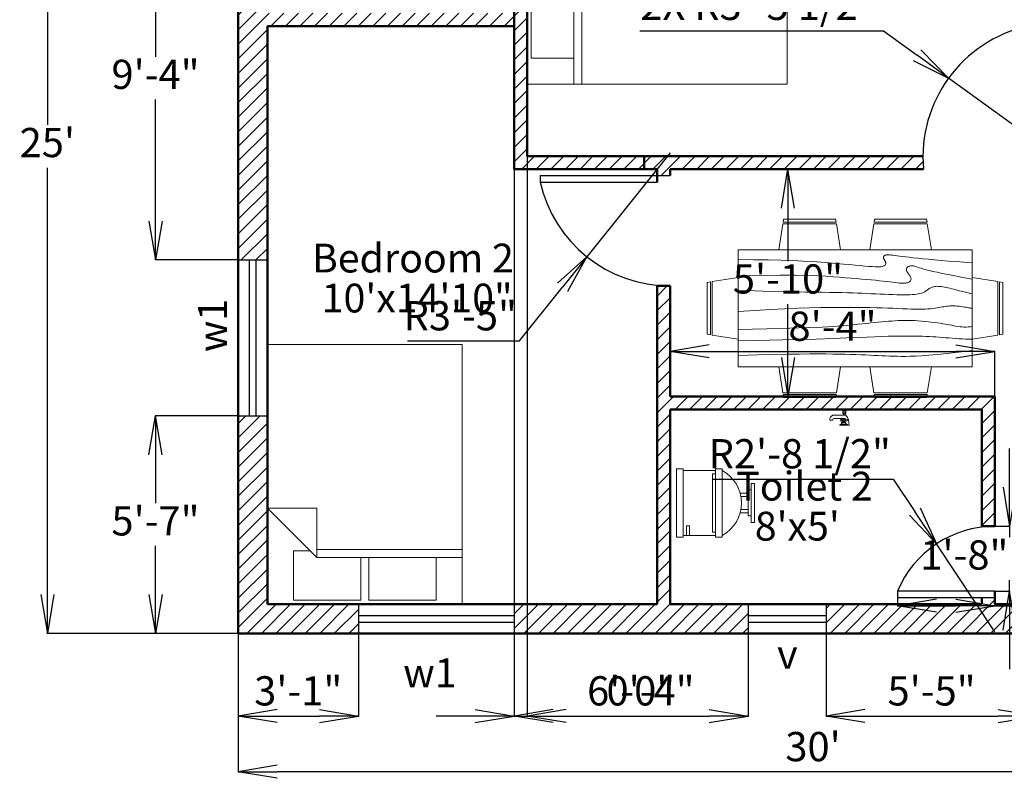
# Model space of a CAD drawing. Units: inches. Extents: x 1856 to 3350, y 1624 to 2224.
# Tile 1 of 7: x 1856 to 2159, y 1782 to 2016. Entities that reach past the tile are written whole.
import ezdxf

# ---------------------------------------------------------------- set-up
doc = ezdxf.new("R2010")
doc.units = ezdxf.units.IN
for name, color, linetype, lineweight in [('A-ANNO-DIMS', 2, 'Continuous', 18), ('A-ANNO-TEXT', 7, 'Continuous', 18), ('A-AREA-IDEN', 7, 'Continuous', 25), ('A-DOOR', 3, 'Continuous', 25), ('A-FLOR-FIXT', 3, 'Continuous', 18), ('A-FURN', 3, 'Continuous', 18), ('A-WALL', 7, 'Continuous', 50), ('A-WALL-PATT', 8, 'Continuous', 13), ('ventilator', 6, 'Continuous', 25), ('window', 4, 'Continuous', 25)]:
    doc.layers.add(name, color=color, linetype=linetype, lineweight=lineweight)
doc.styles.get("Standard").update_dxf_attribs({"font": 'arial.ttf'})
doc.dimstyles.new('ISO-25', dxfattribs={"dimtxt": 9, "dimasz": 12, "dimexe": 0.125, "dimexo": 0.125, "dimgap": 2, "dimtad": 1, "dimtih": 1, "dimtoh": 1, "dimdec": 1, "dimzin": 11, "dimlunit": 4, "dimtxsty": 'Standard', "dimblk": 'OPEN', "dimcen": -0.125, "dimadec": 0, "dimazin": 0, "dimtfac": 1, "dimtdec": 1, "dimtmove": 0, "dimatfit": 3, "dimfxl": 1, "dimarcsym": 0})

# ---------------------------------------------------------------- blocks, each defined once
blk = doc.blocks.new('_Open')
at = {"color": 0, "linetype": 'ByBlock', "lineweight": -2}
for p, q in [((-1, 0.167), (0, 0)), ((-1, -0.167), (0, 0)), ((0, 0), (-1, 0))]:
    blk.add_line(p, q, dxfattribs=at)
blk = doc.blocks.new('*D4')
at = {"layer": 'A-ANNO-DIMS', "color": 0, "lineweight": -2, "transparency": 16777216}
for p, q in [((1922.99, 2126.99), (1864.24, 2126.99)), ((1864.36, 2114.99), (1864.36, 1983.59)), ((1864.36, 1838.99), (1864.36, 1970.4)), ((1922.99, 1826.99), (1864.24, 1826.99))]:
    blk.add_line(p, q, dxfattribs=at)
at = {"layer": 'Defpoints', "color": 0, "transparency": 16777216}
for p in [(1923.11, 2126.99), (1864.36, 1826.99), (1923.11, 1826.99)]:
    blk.add_point(p, dxfattribs=at)
at = {"layer": 'A-ANNO-DIMS', "color": 0, "lineweight": -2, "transparency": 16777216, "xscale": 12, "yscale": 12, "zscale": 12}
for p, rotation in [((1864.36, 2126.99), 90), ((1864.36, 1826.99), 270)]:
    blk.add_blockref('_Open', p, dxfattribs=dict(at, rotation=rotation))
at = {"layer": 'A-ANNO-DIMS', "color": 0, "transparency": 16777216, "insert": (1864.36, 1976.99), "char_height": 9, "attachment_point": 5}
blk.add_mtext("25'", dxfattribs=at)
blk = doc.blocks.new('*D5')
at = {"layer": 'A-ANNO-DIMS', "color": 0, "lineweight": -2, "transparency": 16777216}
for p, q in [((2056.24, 1969.99), (2092.52, 1969.99)), ((2092.4, 1957.99), (2092.4, 1941.59)), ((2092.4, 1911.99), (2092.4, 1928.4)), ((2056.24, 1899.99), (2092.52, 1899.99))]:
    blk.add_line(p, q, dxfattribs=at)
at = {"layer": 'Defpoints', "color": 0, "transparency": 16777216}
for p in [(2056.11, 1969.99), (2056.11, 1899.99), (2092.4, 1899.99)]:
    blk.add_point(p, dxfattribs=at)
at = {"layer": 'A-ANNO-DIMS', "color": 0, "lineweight": -2, "transparency": 16777216, "xscale": 12, "yscale": 12, "zscale": 12}
for p, rotation in [((2092.4, 1969.99), 90), ((2092.4, 1899.99), 270)]:
    blk.add_blockref('_Open', p, dxfattribs=dict(at, rotation=rotation))
at = {"layer": 'A-ANNO-DIMS', "color": 0, "transparency": 16777216, "insert": (2092.4, 1934.99), "char_height": 9, "attachment_point": 5}
blk.add_mtext('5\'-10"', dxfattribs=at)
blk = doc.blocks.new('*D6')
at = {"layer": 'A-ANNO-DIMS', "color": 0, "lineweight": -2, "transparency": 16777216}
for p, q in [((2056.11, 1900.12), (2056.11, 1913.96)), ((2068.11, 1913.84), (2144.11, 1913.84)), ((2156.11, 1900.12), (2156.11, 1913.96))]:
    blk.add_line(p, q, dxfattribs=at)
at = {"layer": 'Defpoints', "color": 0, "transparency": 16777216}
for p in [(2156.11, 1913.84), (2056.11, 1899.99), (2156.11, 1899.99)]:
    blk.add_point(p, dxfattribs=at)
at = {"layer": 'A-ANNO-DIMS', "color": 0, "lineweight": -2, "transparency": 16777216, "xscale": 12, "yscale": 12, "zscale": 12, "rotation": 180}
blk.add_blockref('_Open', (2056.11, 1913.84), dxfattribs=at)
at = {"layer": 'A-ANNO-DIMS', "color": 0, "lineweight": -2, "transparency": 16777216, "xscale": 12, "yscale": 12, "zscale": 12}
blk.add_blockref('_Open', (2156.11, 1913.84), dxfattribs=at)
at = {"layer": 'A-ANNO-DIMS', "color": 0, "transparency": 16777216, "insert": (2106.11, 1920.43), "char_height": 9, "attachment_point": 5}
blk.add_mtext('8\'-4"', dxfattribs=at)
blk = doc.blocks.new('*D7')
at = {"layer": 'A-ANNO-DIMS', "color": 0, "lineweight": -2, "transparency": 16777216}
for p, q in [((1923.11, 1826.87), (1923.11, 1784.25)), ((2277.11, 1826.87), (2277.11, 1784.25)), ((2265.11, 1784.37), (1935.11, 1784.37))]:
    blk.add_line(p, q, dxfattribs=at)
at = {"layer": 'Defpoints', "color": 0, "transparency": 16777216}
for p in [(1923.11, 1826.99), (2277.11, 1826.99), (1923.11, 1784.37)]:
    blk.add_point(p, dxfattribs=at)
at = {"layer": 'A-ANNO-DIMS', "color": 0, "lineweight": -2, "transparency": 16777216, "xscale": 12, "yscale": 12, "zscale": 12, "rotation": 180}
blk.add_blockref('_Open', (1923.11, 1784.37), dxfattribs=at)
at = {"layer": 'A-ANNO-DIMS', "color": 0, "lineweight": -2, "transparency": 16777216, "xscale": 12, "yscale": 12, "zscale": 12}
blk.add_blockref('_Open', (2277.11, 1784.37), dxfattribs=at)
at = {"layer": 'A-ANNO-DIMS', "color": 0, "transparency": 16777216, "insert": (2100.11, 1790.97), "char_height": 9, "attachment_point": 5}
blk.add_mtext("30'", dxfattribs=at)
blk = doc.blocks.new('Bed - Queen')
for p, q in [((0, -80.00003), (0, 0)), ((0, 0), (59.99999, 0)), ((59.99999, 0), (59.99999, -80.00003)), ((7.99999, -1.2), (28.79998, -1.2)), ((7.99999, -14.4), (7.99999, -1.2)), ((28.79998, -1.2), (28.79998, -14.4)), ((31.19999, -1.2), (51.99999, -1.2)), ((31.19999, -14.4), (31.19999, -1.2)), ((51.99999, -1.2), (51.99999, -16.4)), ((0, -14.4), (44.8, -14.4)), ((59.99999, -29.6), (44.8, -14.4)), ((44.8, -14.4), (44.8, -29.6)), ((44.8, -16.8), (0, -16.8)), ((51.99999, -16.4), (46.79936, -16.4)), ((44.8, -29.6), (59.99999, -29.6)), ((59.99999, -80.00003), (0, -80.00003))]:
    blk.add_line(p, q)
blk = doc.blocks.new('Dining Set - 36 x 72 in.')
for p, q in [((-22, 27.5), (-22.1562, 26.50042)), ((-22, 27.5), (-6, 27.5)), ((-5.8437, 26.49966), (-6, 27.5)), ((6, 27.5), (5.8438, 26.50042)), ((6, 27.5), (22, 27.5)), ((22.1563, 26.49966), (22, 27.5)), ((-22.2343, 26.00059), (-23.4847, 17.99762)), ((-22.2304, 26), (-5.7608, 26)), ((-5.8416, 26.5), (-22.1534, 26.5)), ((-4.5152, 17.99762), (-5.7655, 25.99926)), ((5.7657, 26.00059), (4.5153, 17.99762)), ((5.7696, 26), (22.2392, 26)), ((22.1584, 26.5), (5.8466, 26.5)), ((23.4848, 17.99762), (22.2345, 25.99926)), ((36, 18), (-36, 18)), ((-36, 18), (-36, -18)), ((36, -18), (36, 18)), ((-44.0006, 8.23428), (-35.9976, 9.48474)), ((44.0006, 8.23428), (35.9976, 9.48474)), ((-45.5, 8), (-44.5004, 8.15617)), ((-45.5, 8), (-45.5, -8)), ((-44.5, -8.15843), (-44.5, 8.15338)), ((-44, 8.23041), (-44, -8.23915)), ((44, 8.23041), (44, -8.23915)), ((44.5, -8.15843), (44.5, 8.15338)), ((45.5, 8), (44.5005, 8.15617)), ((45.5, 8), (45.5, -8)), ((-44.4997, -8.15631), (-45.5, -8)), ((-35.9976, -9.48476), (-43.9993, -8.2345)), ((35.9976, -9.48476), (43.9993, -8.2345)), ((44.4997, -8.15631), (45.5, -8)), ((-36, -18), (36, -18)), ((-22.2343, -26.0006), (-23.4847, -17.99762)), ((-4.5152, -17.99762), (-5.7655, -25.99928)), ((5.7657, -26.0006), (4.5153, -17.99762)), ((23.4848, -17.99762), (22.2345, -25.99928)), ((-22.2304, -26), (-5.7608, -26)), ((-22, -27.5), (-22.1562, -26.50044)), ((-5.8416, -26.5), (-22.1534, -26.5)), ((-5.8437, -26.49967), (-6, -27.5)), ((5.7696, -26), (22.2392, -26)), ((6, -27.5), (5.8438, -26.50044)), ((22.1584, -26.5), (5.8466, -26.5)), ((22.1563, -26.49967), (22, -27.5)), ((-22, -27.5), (-6, -27.5)), ((6, -27.5), (22, -27.5))]:
    blk.add_line(p, q)
for points in [[(-36, 15), (-31.1772, 14.97754), (-26.8079, 14.91406), (-22.8538, 14.81543), (-19.276, 14.6875), (-16.0362, 14.53613), (-13.0957, 14.36718), (-10.4159, 14.18652), (-7.9583, 14), (-5.6904, 13.81315), (-3.6035, 13.63021), (-1.6954, 13.45508), (0.0365, 13.29166), (1.5945, 13.14388), (2.9811, 13.01562), (4.1988, 12.9108), (5.25, 12.83333), (6.1393, 12.78613), (6.8802, 12.76823), (7.4883, 12.77767), (7.9792, 12.8125), (8.3685, 12.87077), (8.6719, 12.95052), (8.9049, 13.0498), (9.0833, 13.16666), (9.2205, 13.29899), (9.3216, 13.44401), (9.3895, 13.59879), (9.4271, 13.76041), (9.4373, 13.92594), (9.4232, 14.09245), (9.3875, 14.257), (9.3333, 14.41666), (9.2638, 14.56917), (9.1836, 14.71484), (9.0975, 14.85465), (9.0104, 14.98958), (8.9272, 15.1206), (8.8529, 15.2487), (8.7922, 15.37483), (8.75, 15.5), (8.7305, 15.62467), (8.7344, 15.74739), (8.7617, 15.86621), (8.8125, 15.97916), (8.8867, 16.08431), (8.9844, 16.17968), (9.1055, 16.26334), (9.25, 16.33333), (9.4189, 16.38802), (9.6172, 16.42708), (9.8506, 16.45052), (10.125, 16.45833), (10.4463, 16.45052), (10.8203, 16.42708), (11.2529, 16.38802), (11.75, 16.33333), (12.3184, 16.26318), (12.9694, 16.17838), (13.7151, 16.07991), (14.5677, 15.96875), (15.5395, 15.84586), (16.6426, 15.71224), (17.8893, 15.56884), (19.2917, 15.41666), (20.859, 15.25667), (22.5879, 15.08984), (24.4721, 14.91715), (26.5052, 14.73958), (28.6809, 14.5581), (30.9929, 14.3737), (33.4347, 14.18733), (36, 14)], [(-36, 10), (-28.9766, 10.14274), (-23.1725, 10.20442), (-18.4241, 10.19775), (-14.5677, 10.13541), (-11.4399, 10.03011), (-8.877, 9.89453), (-6.7154, 9.74137), (-4.7917, 9.58333), (-2.9698, 9.43082), (-1.2246, 9.28515), (0.4415, 9.14534), (2.026, 9.01041), (3.5266, 8.87939), (4.9408, 8.7513), (6.266, 8.62516), (7.5, 8.5), (8.6411, 8.37549), (9.6914, 8.2539), (10.6538, 8.13818), (11.5312, 8.03125), (12.3267, 7.93603), (13.043, 7.85547), (13.6831, 7.79248), (14.25, 7.75), (14.7471, 7.7303), (15.1797, 7.73307), (15.5537, 7.75732), (15.875, 7.80208), (16.1494, 7.86637), (16.3828, 7.94922), (16.5811, 8.04964), (16.75, 8.16666), (16.8944, 8.29915), (17.0143, 8.44531), (17.1089, 8.60319), (17.1771, 8.77083), (17.218, 8.94629), (17.2305, 9.1276), (17.2137, 9.31282), (17.1667, 9.5), (17.0895, 9.6875), (16.987, 9.875), (16.8649, 10.0625), (16.7292, 10.25), (16.5856, 10.4375), (16.4401, 10.625), (16.2985, 10.8125), (16.1667, 11), (16.05, 11.18733), (15.9518, 11.3737), (15.8752, 11.5581), (15.8229, 11.73958), (15.798, 11.91715), (15.8034, 12.08984), (15.842, 12.25667), (15.9167, 12.41666), (16.0295, 12.56836), (16.1784, 12.70833), (16.3605, 12.83268), (16.5729, 12.9375), (16.8127, 13.01888), (17.0768, 13.07291), (17.3625, 13.0957), (17.6667, 13.08333), (17.9894, 13.03312), (18.3418, 12.94726), (18.7382, 12.82918), (19.1927, 12.68229), (19.7195, 12.51001), (20.3327, 12.31575), (21.0465, 12.10294), (21.875, 11.875), (22.8357, 11.63354), (23.959, 11.37304), (25.2786, 11.08618), (26.8282, 10.76562), (28.6414, 10.40405), (30.752, 9.99414), (33.1936, 9.52856), (36, 9)], [(-36, 5.5), (-30.7157, 5.3348), (-26.069, 5.20963), (-21.9946, 5.11767), (-18.4271, 5.05208), (-15.3009, 5.00602), (-12.5508, 4.97265), (-10.1112, 4.94515), (-7.9167, 4.91666), (-5.909, 4.88167), (-4.0586, 4.83984), (-2.3429, 4.79215), (-0.7396, 4.73958), (0.7739, 4.6831), (2.22, 4.6237), (3.6213, 4.56233), (5, 4.5), (6.373, 4.43782), (7.7344, 4.3776), (9.0723, 4.32129), (10.375, 4.27083), (11.6309, 4.22819), (12.8281, 4.19531), (13.9551, 4.17415), (15, 4.16666), (15.954, 4.17448), (16.819, 4.19791), (17.6001, 4.23698), (18.3021, 4.29166), (18.9299, 4.36198), (19.4883, 4.44791), (19.9823, 4.54948), (20.4167, 4.66666), (20.7969, 4.79899), (21.1302, 4.94401), (21.4245, 5.09879), (21.6875, 5.26041), (21.9271, 5.42594), (22.1511, 5.59245), (22.3672, 5.757), (22.5834, 5.91666), (22.8065, 6.06868), (23.0404, 6.21093), (23.2879, 6.34147), (23.5521, 6.45833), (23.8358, 6.55957), (24.142, 6.64323), (24.4735, 6.70735), (24.8334, 6.75), (25.2235, 6.76969), (25.642, 6.76692), (26.0858, 6.74267), (26.5521, 6.69791), (27.0379, 6.63362), (27.5404, 6.55078), (28.0565, 6.45036), (28.5834, 6.33333), (29.1242, 6.19987), (29.7071, 6.04687), (30.3661, 5.87044), (31.1354, 5.66666), (32.0493, 5.43164), (33.142, 5.16146), (34.4475, 4.85221), (36, 4.5)], [(-36, -1), (-30.7915, -0.6591), (-26.0195, -0.38216), (-21.6519, -0.16284), (-17.6563, 0.00521), (-14.0005, 0.12833), (-10.6523, 0.21289), (-7.5796, 0.26522), (-4.75, 0.29166), (-2.134, 0.29793), (0.2878, 0.28711), (2.5317, 0.26163), (4.6146, 0.22396), (6.5529, 0.17651), (8.3633, 0.12174), (10.0623, 0.06209), (11.6667, 0), (13.1899, -0.06201), (14.6341, -0.1211), (15.9982, -0.17432), (17.2813, -0.21875), (18.4823, -0.25147), (19.6003, -0.26953), (20.6343, -0.27002), (21.5834, -0.25), (22.4481, -0.20768), (23.2357, -0.14584), (23.9549, -0.06836), (24.6146, 0.02083), (25.2235, 0.11784), (25.7904, 0.21875), (26.3241, 0.31966), (26.8334, 0.41666), (27.3265, 0.50618), (27.8099, 0.58593), (28.2894, 0.65397), (28.7709, 0.70833), (29.2601, 0.74707), (29.763, 0.76823), (30.2855, 0.76985), (30.8334, 0.75), (31.4088, 0.70784), (31.9994, 0.64713), (32.589, 0.57275), (33.1615, 0.48958), (33.7008, 0.4025), (34.1908, 0.3164), (34.6153, 0.23616), (34.9584, 0.16666), (35.2099, 0.11165), (35.3848, 0.07031), (35.504, 0.04069), (35.5886, 0.02083), (35.6594, 0.00879), (35.7377, 0.0026), (35.8442, 0.00032), (36, 0)], [(-36, -6.5), (-27.1843, -6.31267), (-20.084, -6.1263), (-14.469, -5.9419), (-10.1094, -5.76042), (-6.7752, -5.58285), (-4.2363, -5.41016), (-2.2629, -5.24333), (-0.625, -5.08334), (0.8708, -4.93099), (2.2715, -4.78646), (3.5872, -4.64974), (4.8281, -4.52084), (6.0046, -4.39974), (7.127, -4.28646), (8.2053, -4.18099), (9.25, -4.08334), (10.2705, -3.99382), (11.2734, -3.91407), (12.2647, -3.84603), (13.25, -3.79167), (14.2354, -3.75293), (15.2266, -3.73177), (16.2295, -3.73015), (17.25, -3.75), (18.2912, -3.79248), (19.3451, -3.85547), (20.4009, -3.93604), (21.4479, -4.03125), (22.4754, -4.13819), (23.4727, -4.25391), (24.4289, -4.37549), (25.3334, -4.5), (26.1785, -4.62492), (26.9694, -4.74935), (27.7145, -4.87281), (28.4219, -4.99479), (29.1, -5.11483), (29.7572, -5.23242), (30.4016, -5.34709), (31.0417, -5.45834), (31.6837, -5.56437), (32.3262, -5.65821), (32.9658, -5.73153), (33.599, -5.77604), (34.2224, -5.78345), (34.8327, -5.74545), (35.4264, -5.65373), (36, -5.5)], [(-36, -10), (-26.4022, -9.81299), (-18.4675, -9.62891), (-11.9839, -9.45069), (-6.7396, -9.28125), (-2.5226, -9.12354), (0.8789, -8.98047), (3.6769, -8.85498), (6.0833, -8.75), (8.2767, -8.66765), (10.3021, -8.60677), (12.1712, -8.56543), (13.8958, -8.54167), (15.4876, -8.53353), (16.9583, -8.53907), (18.3197, -8.55632), (19.5834, -8.58334), (20.7616, -8.61841), (21.8685, -8.66081), (22.9188, -8.71004), (23.9271, -8.76563), (24.9081, -8.82707), (25.8763, -8.89388), (26.8465, -8.96558), (27.8334, -9.04167), (28.8474, -9.12118), (29.8828, -9.20117), (30.93, -9.27824), (31.9792, -9.34896), (33.0205, -9.40991), (34.0443, -9.45768), (35.0407, -9.48885), (36, -9.5)], [(-36, -14.5), (-30.0881, -14.33513), (-25.0332, -14.21224), (-20.7312, -14.12647), (-17.0781, -14.07292), (-13.97, -14.04671), (-11.3027, -14.04297), (-8.9724, -14.05681), (-6.875, -14.08334), (-4.9224, -14.11833), (-3.0905, -14.16016), (-1.3709, -14.20785), (0.2448, -14.26042), (1.7647, -14.3169), (3.1973, -14.3763), (4.5507, -14.43767), (5.8333, -14.5), (7.0554, -14.5621), (8.235, -14.62175), (9.3922, -14.67652), (10.5469, -14.72396), (11.7192, -14.76164), (12.929, -14.78711), (14.1965, -14.79794), (15.5417, -14.79167), (16.9933, -14.76424), (18.6152, -14.70508), (20.4804, -14.60197), (22.6615, -14.44271), (25.2312, -14.21509), (28.2624, -13.9069), (31.8277, -13.50594), (36, -13)]]:
    blk.add_lwpolyline(points)
blk = doc.blocks.new('Toilet - front')
for p, q in [((-10, 22), (-10, 12)), ((10, 12), (10, 22)), ((-10, 21), (-7, 21)), ((-7, 20), (-10, 20)), ((-7, 21), (-7, 20)), ((9, 13), (-9, 13)), ((-9, 13), (-9, 12)), ((9, 12), (9, 13)), ((10.5, 12), (-10.5, 12)), ((-10.5, 10), (-10.5, 12)), ((10.5, 10), (-10.5, 10)), ((10.5, 12), (10.5, 10)), ((-3, 4.4065), (-3, 2)), ((-2, 2), (-2, 4.1658)), ((2, 4.1658), (2, 2)), ((3, 2), (3, 4.4065)), ((4, 2), (-4, 2)), ((-4, 2), (-4, 1)), ((4, 1), (4, 2))]:
    blk.add_line(p, q)
for points in [[(10.5, 22), (10.5, 24), (-10.5, 24), (-10.5, 22)], [(6, 0), (6, 1), (-6, 1), (-6, 0)]]:
    blk.add_lwpolyline(points, close=True)
blk.add_arc((0, 15.3333), 11.3333, 208.0725, 331.9275)
blk = doc.blocks.new('Faucet - Bathroom side')
for p, q in [((-0.625, 4.25), (0.375, 4.25)), ((0.375, 3.75), (-0.625, 3.75)), ((-0.375, 3), (-0.375, 3.5)), ((0.125, 3.5), (0.125, 3)), ((-1.625, 0), (-1.375, 0)), ((-1.375, 0), (1.375, 0)), ((-0.88366, 0.25), (0.88424, 0.25)), ((-0.625, 3), (3.375, 3)), ((-0.375, 1.625), (-0.625, 1.625)), ((-0.375, 1.375), (-0.625, 1.375)), ((0.48078, 0.75), (-0.47286, 0.75)), ((2.875, 2), (0.375, 2)), ((0.375, 1.625), (0.625, 1.625)), ((0.375, 1.375), (0.625, 1.375)), ((4.375, 1.5), (3.375, 1.5))]:
    blk.add_line(p, q)
for points in [[(-0.625, 3.75), (-0.625, 4.25)], [(-0.375, 4.5), (0.125, 4.5)], [(0.125, 3.5), (-0.375, 3.5)], [(0.375, 4.25), (0.375, 3.75)]]:
    blk.add_lwpolyline(points)
blk.add_lwpolyline([(-0.375, 1), (-0.375, 2), (0.375, 2), (0.375, 1)], close=True)
for centre in [(-0.875, 1.5), (0, 1.5), (0.875, 1.5)]:
    blk.add_circle(centre, 0.27951)
for centre, radius, start, end in [((-0.38253, 4.2575), 0.24259, 88.22243, 181.7776), ((-0.38253, 3.7424), 0.24259, 178.2224, 271.7776), ((0.13252, 4.2575), 0.24259, 358.2224, 91.77757), ((0.13252, 3.7424), 0.24259, 268.2224, 1.777565), ((3.45929, -0.0281), 5.08436, 143.4467, 179.6834), ((-1.75, 1.375), 1.42522, 285.2551, 344.7449), ((1.75, 1.375), 1.42522, 195.2551, 254.7449), ((-2.49562, -0.286), 3.38273, 9.709485, 29.48735), ((2.96867, 1.5936), 0.41699, 347.0192, 102.9808), ((2.70708, 1.4714), 1.66816, 0.9827695, 66.39737)]:
    blk.add_arc(centre, radius, start, end)
blk = doc.blocks.new('WIN-48')
for p, q in [((0, 9), (48, 9)), ((0, 9), (0, 0)), ((48, 9), (48, 0)), ((0, 5.5), (48, 5.5)), ((0, 3.5), (48, 3.5)), ((0, 0), (48, 0))]:
    blk.add_line(p, q)
blk = doc.blocks.new('VENT-24')
for p, q in [((0, 9), (24, 9)), ((0, 9), (0, 0)), ((24, 9), (24, 0)), ((0, 5.5), (24, 5.5)), ((0, 3.5), (24, 3.5)), ((0, 0), (24, 0))]:
    blk.add_line(p, q)
blk = doc.blocks.new('DOOR-SWING-44')
blk.add_line((32.16, 44), (32.16, 0))
blk.add_arc((41.37, 3.67), 41.37, 102.8606, 185.0846)
blk = doc.blocks.new('DOOR-SWING-30')
blk.add_line((30, 0), (0, 0))
blk.add_arc((30, -12.5), 32.5, 90, 157.3801)
blk = doc.blocks.new('*D60')
at = {"layer": 'A-ANNO-DIMS', "color": 0, "lineweight": -2, "transparency": 16777216}
for p, q in [((2126.11, 1839.87), (2126.11, 1835.37)), ((2156.11, 1839.87), (2156.11, 1835.37)), ((2138.11, 1835.49), (2144.11, 1835.49)), ((2156.11, 1835.49), (2313.84, 1835.49))]:
    blk.add_line(p, q, dxfattribs=at)
at = {"layer": 'Defpoints', "color": 0, "transparency": 16777216}
for p in [(2126.11, 1839.99), (2156.11, 1839.99), (2156.11, 1835.49)]:
    blk.add_point(p, dxfattribs=at)
at = {"layer": 'A-ANNO-DIMS', "color": 0, "lineweight": -2, "transparency": 16777216, "xscale": 12, "yscale": 12, "zscale": 12, "rotation": 180}
blk.add_blockref('_Open', (2126.11, 1835.49), dxfattribs=at)
at = {"layer": 'A-ANNO-DIMS', "color": 0, "lineweight": -2, "transparency": 16777216, "xscale": 12, "yscale": 12, "zscale": 12}
blk.add_blockref('_Open', (2156.11, 1835.49), dxfattribs=at)
at = {"layer": 'A-ANNO-DIMS', "color": 0, "transparency": 16777216, "insert": (2240.97, 1842.15), "char_height": 9, "attachment_point": 5}
blk.add_mtext('DOOR SWING 2\'-6" TYP.', dxfattribs=at)
blk = doc.blocks.new('*D61')
at = {"layer": 'A-ANNO-DIMS', "color": 0, "lineweight": -2, "transparency": 16777216}
for p, q in [((2160.61, 1871.99), (2160.61, 1883.99)), ((2156.24, 1859.99), (2160.74, 1859.99)), ((2160.61, 1859.99), (2160.61, 1856.59)), ((2160.61, 1839.99), (2160.61, 1843.4)), ((2156.24, 1839.99), (2160.74, 1839.99)), ((2160.61, 1827.99), (2160.61, 1815.99))]:
    blk.add_line(p, q, dxfattribs=at)
at = {"layer": 'Defpoints', "color": 0, "transparency": 16777216}
for p in [(2156.11, 1859.99), (2160.61, 1859.99), (2156.11, 1839.99)]:
    blk.add_point(p, dxfattribs=at)
at = {"layer": 'A-ANNO-DIMS', "color": 0, "lineweight": -2, "transparency": 16777216, "xscale": 12, "yscale": 12, "zscale": 12}
for p, rotation in [((2160.61, 1859.99), 270), ((2160.61, 1839.99), 90)]:
    blk.add_blockref('_Open', p, dxfattribs=dict(at, rotation=rotation))
at = {"layer": 'A-ANNO-DIMS', "color": 0, "transparency": 16777216, "insert": (2160.61, 1849.99), "char_height": 9, "attachment_point": 5}
blk.add_mtext('1\'-8" TYP.', dxfattribs=at)
blk = doc.blocks.new('*D68')
at = {"layer": 'A-ANNO-DIMS', "color": 0, "lineweight": -2, "transparency": 16777216}
for p, q in [((1923.11, 1826.87), (1923.11, 1801.42)), ((1960.11, 1826.87), (1960.11, 1801.42)), ((1935.11, 1801.54), (1948.11, 1801.54))]:
    blk.add_line(p, q, dxfattribs=at)
at = {"layer": 'Defpoints', "color": 0, "transparency": 16777216}
for p in [(1923.11, 1826.99), (1960.11, 1826.99), (1960.11, 1801.54)]:
    blk.add_point(p, dxfattribs=at)
at = {"layer": 'A-ANNO-DIMS', "color": 0, "lineweight": -2, "transparency": 16777216, "xscale": 12, "yscale": 12, "zscale": 12, "rotation": 180}
blk.add_blockref('_Open', (1923.11, 1801.54), dxfattribs=at)
at = {"layer": 'A-ANNO-DIMS', "color": 0, "lineweight": -2, "transparency": 16777216, "xscale": 12, "yscale": 12, "zscale": 12}
blk.add_blockref('_Open', (1960.11, 1801.54), dxfattribs=at)
at = {"layer": 'A-ANNO-DIMS', "color": 0, "transparency": 16777216, "insert": (1941.61, 1808.14), "char_height": 9, "attachment_point": 5}
blk.add_mtext('3\'-1"', dxfattribs=at)
blk = doc.blocks.new('*D69')
at = {"layer": 'A-ANNO-DIMS', "color": 0, "lineweight": -2, "transparency": 16777216}
for p, q in [((2008.11, 1826.87), (2008.11, 1801.42)), ((2080.11, 1826.87), (2080.11, 1801.42)), ((2020.11, 1801.54), (2068.11, 1801.54))]:
    blk.add_line(p, q, dxfattribs=at)
at = {"layer": 'Defpoints', "color": 0, "transparency": 16777216}
for p in [(2008.11, 1826.99), (2080.11, 1826.99), (2080.11, 1801.54)]:
    blk.add_point(p, dxfattribs=at)
at = {"layer": 'A-ANNO-DIMS', "color": 0, "lineweight": -2, "transparency": 16777216, "xscale": 12, "yscale": 12, "zscale": 12, "rotation": 180}
blk.add_blockref('_Open', (2008.11, 1801.54), dxfattribs=at)
at = {"layer": 'A-ANNO-DIMS', "color": 0, "lineweight": -2, "transparency": 16777216, "xscale": 12, "yscale": 12, "zscale": 12}
blk.add_blockref('_Open', (2080.11, 1801.54), dxfattribs=at)
at = {"layer": 'A-ANNO-DIMS', "color": 0, "transparency": 16777216, "insert": (2044.11, 1808.14), "char_height": 9, "attachment_point": 5}
blk.add_mtext('6\'-0"', dxfattribs=at)
blk = doc.blocks.new('*D70')
at = {"layer": 'A-ANNO-DIMS', "color": 0, "lineweight": -2, "transparency": 16777216}
for p, q in [((2104.11, 1826.87), (2104.11, 1801.42)), ((2169.11, 1826.87), (2169.11, 1801.42)), ((2116.11, 1801.54), (2157.11, 1801.54))]:
    blk.add_line(p, q, dxfattribs=at)
at = {"layer": 'Defpoints', "color": 0, "transparency": 16777216}
for p in [(2104.11, 1826.99), (2169.11, 1826.99), (2169.11, 1801.54)]:
    blk.add_point(p, dxfattribs=at)
at = {"layer": 'A-ANNO-DIMS', "color": 0, "lineweight": -2, "transparency": 16777216, "xscale": 12, "yscale": 12, "zscale": 12, "rotation": 180}
blk.add_blockref('_Open', (2104.11, 1801.54), dxfattribs=at)
at = {"layer": 'A-ANNO-DIMS', "color": 0, "lineweight": -2, "transparency": 16777216, "xscale": 12, "yscale": 12, "zscale": 12}
blk.add_blockref('_Open', (2169.11, 1801.54), dxfattribs=at)
at = {"layer": 'A-ANNO-DIMS', "color": 0, "transparency": 16777216, "insert": (2136.61, 1808.12), "char_height": 9, "attachment_point": 5}
blk.add_mtext('5\'-5"', dxfattribs=at)
blk = doc.blocks.new('*D71')
at = {"layer": 'A-ANNO-DIMS', "color": 0, "lineweight": -2, "transparency": 16777216}
for p, q in [((1922.99, 1893.99), (1897.54, 1893.99)), ((1897.66, 1881.99), (1897.66, 1867.07)), ((1897.66, 1838.99), (1897.66, 1853.92)), ((1922.99, 1826.99), (1897.54, 1826.99))]:
    blk.add_line(p, q, dxfattribs=at)
at = {"layer": 'Defpoints', "color": 0, "transparency": 16777216}
for p in [(1897.66, 1893.99), (1923.11, 1893.99), (1923.11, 1826.99)]:
    blk.add_point(p, dxfattribs=at)
at = {"layer": 'A-ANNO-DIMS', "color": 0, "lineweight": -2, "transparency": 16777216, "xscale": 12, "yscale": 12, "zscale": 12}
for p, rotation in [((1897.66, 1893.99), 90), ((1897.66, 1826.99), 270)]:
    blk.add_blockref('_Open', p, dxfattribs=dict(at, rotation=rotation))
at = {"layer": 'A-ANNO-DIMS', "color": 0, "transparency": 16777216, "insert": (1897.66, 1860.49), "char_height": 9, "attachment_point": 5}
blk.add_mtext('5\'-7"', dxfattribs=at)
blk = doc.blocks.new('*D72')
at = {"layer": 'A-ANNO-DIMS', "color": 0, "lineweight": -2, "transparency": 16777216}
for p, q in [((1922.99, 2053.99), (1897.54, 2053.99)), ((1897.66, 2041.99), (1897.66, 2004.59)), ((1897.66, 1953.99), (1897.66, 1991.4)), ((1922.99, 1941.99), (1897.54, 1941.99))]:
    blk.add_line(p, q, dxfattribs=at)
at = {"layer": 'Defpoints', "color": 0, "transparency": 16777216}
for p in [(1897.66, 2053.99), (1923.11, 2053.99), (1923.11, 1941.99)]:
    blk.add_point(p, dxfattribs=at)
at = {"layer": 'A-ANNO-DIMS', "color": 0, "lineweight": -2, "transparency": 16777216, "xscale": 12, "yscale": 12, "zscale": 12}
for p, rotation in [((1897.66, 2053.99), 90), ((1897.66, 1941.99), 270)]:
    blk.add_blockref('_Open', p, dxfattribs=dict(at, rotation=rotation))
at = {"layer": 'A-ANNO-DIMS', "color": 0, "transparency": 16777216, "insert": (1897.66, 1997.99), "char_height": 9, "attachment_point": 5}
blk.add_mtext('9\'-4"', dxfattribs=at)
blk = doc.blocks.new('*D74')
at = {"layer": 'A-ANNO-DIMS', "color": 0, "lineweight": -2, "transparency": 16777216}
for p, q in [((2012.11, 1973.87), (2012.11, 1801.42)), ((2008.11, 1969.87), (2008.11, 1801.42)), ((1996.11, 1801.54), (1984.11, 1801.54)), ((2008.11, 1801.54), (2012.11, 1801.54)), ((2024.11, 1801.54), (2064.04, 1801.54))]:
    blk.add_line(p, q, dxfattribs=at)
at = {"layer": 'Defpoints', "color": 0, "transparency": 16777216}
for p in [(2012.11, 1973.99), (2008.11, 1969.99), (2012.11, 1801.54)]:
    blk.add_point(p, dxfattribs=at)
at = {"layer": 'A-ANNO-DIMS', "color": 0, "lineweight": -2, "transparency": 16777216, "xscale": 12, "yscale": 12, "zscale": 12}
blk.add_blockref('_Open', (2008.11, 1801.54), dxfattribs=at)
at = {"layer": 'A-ANNO-DIMS', "color": 0, "lineweight": -2, "transparency": 16777216, "xscale": 12, "yscale": 12, "zscale": 12, "rotation": 180}
blk.add_blockref('_Open', (2012.11, 1801.54), dxfattribs=at)
at = {"layer": 'A-ANNO-DIMS', "color": 0, "transparency": 16777216, "insert": (2050.08, 1808.14), "char_height": 9, "attachment_point": 5}
blk.add_mtext('0\'-4"', dxfattribs=at)
blk = doc.blocks.new('*D90')
at = {"layer": 'A-ANNO-DIMS', "color": 0, "lineweight": -2, "transparency": 16777216}
for p, q in [((2056.11, 1974.99), (2030.5, 1942.98)), ((2009.76, 1917.06), (2023, 1933.61)), ((1975.23, 1917.06), (2009.76, 1917.06))]:
    blk.add_line(p, q, dxfattribs=at)
at = {"layer": 'Defpoints', "color": 0, "transparency": 16777216}
for p in [(2056.11, 1974.99), (2030.5, 1942.98)]:
    blk.add_point(p, dxfattribs=at)
at = {"layer": 'A-ANNO-DIMS', "color": 0, "lineweight": -2, "transparency": 16777216, "xscale": 12, "yscale": 12, "zscale": 12, "rotation": 51.34046389901789}
blk.add_blockref('_Open', (2030.5, 1942.98), dxfattribs=at)
at = {"layer": 'A-ANNO-DIMS', "color": 0, "transparency": 16777216, "insert": (1991.49, 1923.65), "char_height": 9, "attachment_point": 5}
blk.add_mtext('R3\'-5"', dxfattribs=at)
blk = doc.blocks.new('*D91')
at = {"layer": 'A-ANNO-DIMS', "color": 0, "lineweight": -2, "transparency": 16777216}
for p, q in [((2046.79, 2012.59), (2121.79, 2012.59)), ((2121.79, 2012.59), (2132.16, 2005.05)), ((2175.32, 1973.66), (2141.86, 1997.99))]:
    blk.add_line(p, q, dxfattribs=at)
at = {"layer": 'Defpoints', "color": 0, "transparency": 16777216}
for p in [(2141.86, 1997.99), (2175.32, 1973.66)]:
    blk.add_point(p, dxfattribs=at)
at = {"layer": 'A-ANNO-DIMS', "color": 0, "lineweight": -2, "transparency": 16777216, "xscale": 12, "yscale": 12, "zscale": 12, "rotation": 323.9723172818348}
blk.add_blockref('_Open', (2141.86, 1997.99), dxfattribs=at)
at = {"layer": 'A-ANNO-DIMS', "color": 0, "transparency": 16777216, "insert": (2083.29, 2019.25), "char_height": 9, "attachment_point": 5}
blk.add_mtext('2X R3\'-5 1/2"', dxfattribs=at)
blk = doc.blocks.new('*D92')
at = {"layer": 'A-ANNO-DIMS', "color": 0, "lineweight": -2, "transparency": 16777216}
for p, q in [((2069.26, 1874.5), (2124.77, 1874.5)), ((2124.77, 1874.5), (2131.43, 1864.52)), ((2156.11, 1827.49), (2138.09, 1854.53))]:
    blk.add_line(p, q, dxfattribs=at)
at = {"layer": 'Defpoints', "color": 0, "transparency": 16777216}
for p in [(2138.09, 1854.53), (2156.11, 1827.49)]:
    blk.add_point(p, dxfattribs=at)
at = {"layer": 'A-ANNO-DIMS', "color": 0, "lineweight": -2, "transparency": 16777216, "xscale": 12, "yscale": 12, "zscale": 12, "rotation": 303.6909344406329}
blk.add_blockref('_Open', (2138.09, 1854.53), dxfattribs=at)
at = {"layer": 'A-ANNO-DIMS', "color": 0, "transparency": 16777216, "insert": (2096.02, 1881.16), "char_height": 9, "attachment_point": 5}
blk.add_mtext('R2\'-8 1/2"', dxfattribs=at)

msp = doc.modelspace()

# ---------------------------------------------------------------- hatches: boundary and pattern name
at = {"layer": 'A-WALL-PATT'}
h = msp.add_hatch(dxfattribs=at)
h.set_pattern_fill('ANSI31', color=256)
h.paths.add_polyline_path([(2210.14, 2126.99), (2096.3, 2126.99), (2096.3, 2117.99), (2210.14, 2117.99)])
h.paths.add_polyline_path([(2048.3, 2126.99), (1923.11, 2126.99), (1923.11, 2077.99), (1932.11, 2077.99), (1932.11, 2117.99), (2006.11, 2117.99), (2008.11, 2117.99), (2008.11, 2113.99), (2012.11, 2113.99), (2012.11, 2117.99), (2048.29, 2117.99)])
h.paths.add_polyline_path([(2277.11, 2126.99), (2234.14, 2126.99), (2234.14, 2117.99), (2268.11, 2117.99), (2268.11, 1997.99), (2266.11, 1997.99), (2266.11, 1993.99), (2268.11, 1993.99), (2268.11, 1937.99), (2277.11, 1937.99)])
h.paths.add_polyline_path([(2277.11, 1887.99), (2268.11, 1887.99), (2268.11, 1835.99), (2229.11, 1835.99), (2229.11, 1826.99), (2277.11, 1826.99)])
h.paths.add_polyline_path([(2056.11, 1895.99), (2152.11, 1895.99), (2152.11, 1859.99), (2156.11, 1859.99), (2156.11, 1899.99), (2056.11, 1899.99), (2056.11, 1933.99), (2052.11, 1933.99), (2052.11, 1835.99), (2008.11, 1835.99), (2008.11, 1826.99), (2080.11, 1826.99), (2080.11, 1835.99), (2056.11, 1835.99)])
h.paths.add_polyline_path([(2169.11, 1835.99), (2156.11, 1835.99), (2156.11, 1837.99), (2152.11, 1837.99), (2152.11, 1835.99), (2104.11, 1835.99), (2104.11, 1826.99), (2169.11, 1826.99)])
h.paths.add_polyline_path([(1932.11, 1893.99), (1923.11, 1893.99), (1923.11, 1826.99), (1960.11, 1826.99), (1960.11, 1835.99), (1932.11, 1835.99)])
h.paths.add_polyline_path([(1932.11, 2013.99), (2008.11, 2013.99), (2008.11, 2017.99), (1932.11, 2017.99), (1932.11, 2053.99), (1923.11, 2053.99), (1923.11, 1941.99), (1932.11, 1941.99)])
h.paths.add_polyline_path([(2012.11, 2093.99, -0.030857), (2008.11, 2094.24), (2008.11, 1969.99), (2048.11, 1969.99), (2048.12, 1973.99), (2012.11, 1973.99)])
h.paths.add_polyline_path([(2172.11, 2117.99), (2168.11, 2117.99), (2168.11, 1969.99), (2172.11, 1969.99), (2172.11, 1993.99), (2234.11, 1993.99, -0.024205), (2233.95, 1997.99), (2172.11, 1997.99)])
h.paths.add_polyline_path([(2133.95, 1973.99), (2048.12, 1973.99), (2048.11, 1969.99), (2052.11, 1969.99), (2052.11, 1967.99), (2056.11, 1967.99), (2056.11, 1969.99), (2134.11, 1969.99, -0.024205)])

# ---------------------------------------------------------------- linework, layer by layer
at = {"layer": 'A-DOOR'}
for p, q in [((2016.11, 1967.99), (2016.11, 1965.99)), ((2016.11, 1967.99), (2056.11, 1967.99)), ((2016.11, 1965.99), (2052.11, 1965.99)), ((2126.11, 1839.99), (2126.11, 1837.99)), ((2156.11, 1837.99), (2126.11, 1837.99))]:
    msp.add_line(p, q, dxfattribs=at)
msp.add_arc((2056.11, 1974.99), 41, 192.6804, 270, dxfattribs=at)
at = {"layer": 'A-WALL'}
for p, q in [((1923.11, 2126.99), (1923.11, 1826.99)), ((2008.11, 2093.99), (2008.11, 1969.99)), ((2012.11, 2093.99), (2012.11, 1973.99)), ((1932.11, 2013.99), (1932.11, 1835.99)), ((2008.11, 2013.99), (1932.11, 2013.99)), ((2012.11, 1973.99), (2133.95, 1973.99)), ((2048.12, 1973.99), (2048.11, 1970.14)), ((2008.11, 1969.99), (2052.11, 1969.99)), ((2052.11, 1969.99), (2052.11, 1965.99)), ((2056.11, 1969.99), (2056.11, 1967.99)), ((2056.11, 1969.99), (2134.11, 1969.99)), ((2052.11, 1933.99), (2056.11, 1933.99)), ((2052.11, 1933.99), (2052.11, 1835.99)), ((2056.11, 1933.99), (2056.11, 1899.99)), ((2156.11, 1899.99), (2056.11, 1899.99)), ((2156.11, 1899.99), (2156.11, 1859.99)), ((2152.11, 1895.99), (2056.11, 1895.99)), ((2056.11, 1895.99), (2056.11, 1835.99)), ((2152.11, 1895.99), (2152.11, 1859.99)), ((2156.11, 1859.99), (2152.11, 1859.99)), ((2152.11, 1837.99), (2152.11, 1835.99)), ((2156.11, 1839.99), (2156.11, 1835.99)), ((2052.11, 1835.99), (1932.11, 1835.99)), ((2152.11, 1835.99), (2056.11, 1835.99)), ((2268.11, 1835.99), (2156.11, 1835.99)), ((2277.11, 1826.99), (1923.11, 1826.99))]:
    msp.add_line(p, q, dxfattribs=at)
at = {"layer": 'ventilator'}
msp.add_line((2104.11, 1835.99), (2104.11, 1826.99), dxfattribs=at)

# ---------------------------------------------------------------- block references
at = {"layer": 'A-DOOR'}
for name, p in [('DOOR-SWING-44', (2133.95, 1969.99)), ('DOOR-SWING-30', (2126.11, 1839.99))]:
    msp.add_blockref(name, p, dxfattribs=at)
at = {"layer": 'A-FLOR-FIXT', "xscale": -1}
msp.add_blockref('Faucet - Bathroom side', (2109.62, 1891.16), dxfattribs=at)
at = {"layer": 'A-FLOR-FIXT', "rotation": 90}
msp.add_blockref('Toilet - front', (2082.11, 1867.16), dxfattribs=at)
at = {"layer": 'A-FURN'}
for p, rotation in [((2012.11, 1996.1), 90), ((1992.11, 1835.99), 180)]:
    msp.add_blockref('Bed - Queen', p, dxfattribs=dict(at, rotation=rotation))
msp.add_blockref('Dining Set - 36 x 72 in.', (2113.06, 1927.11), dxfattribs=at)
at = {"layer": 'ventilator'}
msp.add_blockref('VENT-24', (2080.11, 1826.99), dxfattribs=at)
at = {"layer": 'window', "rotation": 89.9999999999994}
msp.add_blockref('WIN-48', (1932.11, 1893.99), dxfattribs=at)
at = {"layer": 'window'}
msp.add_blockref('WIN-48', (1960.11, 1826.99), dxfattribs=at)

# ---------------------------------------------------------------- texts
at = {"layer": 'A-ANNO-TEXT'}
msp.add_text('w1', height=8.871, rotation=90, dxfattribs=at).set_placement((1919.63, 1913.61))
for s, height, p in [('v', 8.87, (2089.06, 1816.1)), ('w1', 8.871, (1973.93, 1810.43))]:
    msp.add_text(s, height=height, dxfattribs=at).set_placement(p)
at = {"layer": 'A-AREA-IDEN'}
for s, height, p in [('Bedroom 2', 8.871, (1945.83, 1938.15)), ('  10\'x14\'10"', 8.8713, (1943.41, 1925.83)), (' Toilet 2', 8.871, (2073.75, 1867.9)), ("    8'x5'", 8.871, (2071.33, 1855.58))]:
    msp.add_text(s, height=height, dxfattribs=at).set_placement(p)

# ---------------------------------------------------------------- dimensions: what is measured, and where the dimension line sits
at = {"layer": 'A-ANNO-DIMS'}
for base, p1, p2, text, override, picture, middle in [((1864.36, 1826.99), (1923.11, 2126.99), (1923.11, 1826.99), "25'", {"dimclrd": 0, "dimclre": 0, "dimclrt": 0}, '*D4', (1864.36, 1976.99)), ((2160.61, 1859.99), (2156.11, 1839.99), (2156.11, 1859.99), '<> TYP.', {"dimdec": 1, "dimlfac": 1, "dimrnd": 0, "dimzin": 1, "dimdsep": 46, "dimlunit": 4, "dimfrac": 2}, '*D61', (2160.61, 1849.99))]:
    dim = msp.add_linear_dim(base=base, p1=p1, p2=p2, angle=90, text=text, dimstyle='ISO-25', override=override, dxfattribs=at)
    dim.commit()
    dim.dimension.update_dxf_attribs({"geometry": picture, "text_midpoint": middle})
for base, p1, p2, override, picture, middle in [((1897.66, 2053.99), (1923.11, 1941.99), (1923.11, 2053.99), {"dimdec": 1, "dimlfac": 1, "dimrnd": 0, "dimzin": 1, "dimdsep": 46, "dimlunit": 4, "dimfrac": 2}, '*D72', (1897.66, 1997.99)), ((2092.4, 1899.99), (2056.11, 1969.99), (2056.11, 1899.99), {"dimclrd": 0, "dimclre": 0, "dimclrt": 0}, '*D5', (2092.4, 1934.99)), ((1897.66, 1893.99), (1923.11, 1826.99), (1923.11, 1893.99), {"dimdec": 1, "dimlfac": 1, "dimrnd": 0, "dimzin": 1, "dimdsep": 46, "dimlunit": 4, "dimfrac": 2}, '*D71', (1897.66, 1860.49))]:
    dim = msp.add_linear_dim(base=base, p1=p1, p2=p2, angle=90, dimstyle='ISO-25', override=override, dxfattribs=at)
    dim.commit()
    dim.dimension.update_dxf_attribs({"geometry": picture, "text_midpoint": middle})
dim = msp.add_radius_dim(center=(2175.32, 1973.66), mpoint=(2141.86, 1997.99), text='2X <>', dimstyle='ISO-25', override={"dimdec": 1, "dimlfac": 1, "dimrnd": 0, "dimzin": 1, "dimdsep": 46, "dimlunit": 4, "dimfrac": 2}, dxfattribs=at)
dim.commit()
dim.dimension.update_dxf_attribs({"geometry": '*D91', "text_midpoint": (2083.29, 2012.59), "dimtype": 164})
for center, mpoint, picture, middle in [((2056.11, 1974.99), (2030.5, 1942.98), '*D90', (1991.49, 1923.65)), ((2156.11, 1827.49), (2138.09, 1854.53), '*D92', (2096.02, 1881.16))]:
    dim = msp.add_radius_dim(center=center, mpoint=mpoint, dimstyle='ISO-25', override={"dimdec": 1, "dimlfac": 1, "dimrnd": 0, "dimzin": 1, "dimdsep": 46, "dimlunit": 4, "dimfrac": 2}, dxfattribs=at)
    dim.commit()
    dim.dimension.update_dxf_attribs({"geometry": picture, "text_midpoint": middle})
for base, p1, p2, override, picture, middle in [((2012.11, 1801.54), (2008.11, 1969.99), (2012.11, 1973.99), {"dimdec": 1, "dimlfac": 1, "dimrnd": 0, "dimzin": 1, "dimdsep": 46, "dimlunit": 4, "dimfrac": 2}, '*D74', (2050.08, 1808.14)), ((2156.11, 1913.84), (2056.11, 1899.99), (2156.11, 1899.99), {"dimclrd": 0, "dimclre": 0, "dimclrt": 0}, '*D6', (2106.11, 1920.43)), ((1960.11, 1801.54), (1923.11, 1826.99), (1960.11, 1826.99), {"dimdec": 1, "dimlfac": 1, "dimrnd": 0, "dimzin": 1, "dimdsep": 46, "dimlunit": 4, "dimfrac": 2}, '*D68', (1941.61, 1808.14)), ((2080.11, 1801.54), (2008.11, 1826.99), (2080.11, 1826.99), {"dimdec": 1, "dimlfac": 1, "dimrnd": 0, "dimzin": 1, "dimdsep": 46, "dimlunit": 4, "dimfrac": 2}, '*D69', (2044.11, 1808.14)), ((2169.11, 1801.54), (2104.11, 1826.99), (2169.11, 1826.99), {"dimdec": 1, "dimlfac": 1, "dimrnd": 0, "dimzin": 1, "dimdsep": 46, "dimlunit": 4, "dimfrac": 2}, '*D70', (2136.61, 1808.12))]:
    dim = msp.add_linear_dim(base=base, p1=p1, p2=p2, dimstyle='ISO-25', override=override, dxfattribs=at)
    dim.commit()
    dim.dimension.update_dxf_attribs({"geometry": picture, "text_midpoint": middle})
for base, p1, p2, text, override, picture, middle in [((2156.11, 1835.49), (2126.11, 1839.99), (2156.11, 1839.99), 'DOOR SWING <> TYP.', {"dimdec": 1, "dimlfac": 1, "dimrnd": 0, "dimzin": 1, "dimdsep": 46, "dimlunit": 4, "dimfrac": 2}, '*D60', (2240.97, 1842.15)), ((1923.11, 1784.37), (2277.11, 1826.99), (1923.11, 1826.99), "30'", {"dimclrd": 0, "dimclre": 0, "dimclrt": 0}, '*D7', (2100.11, 1790.97))]:
    dim = msp.add_linear_dim(base=base, p1=p1, p2=p2, text=text, dimstyle='ISO-25', override=override, dxfattribs=at)
    dim.commit()
    dim.dimension.update_dxf_attribs({"geometry": picture, "text_midpoint": middle})

doc.saveas('drawing.dxf')
